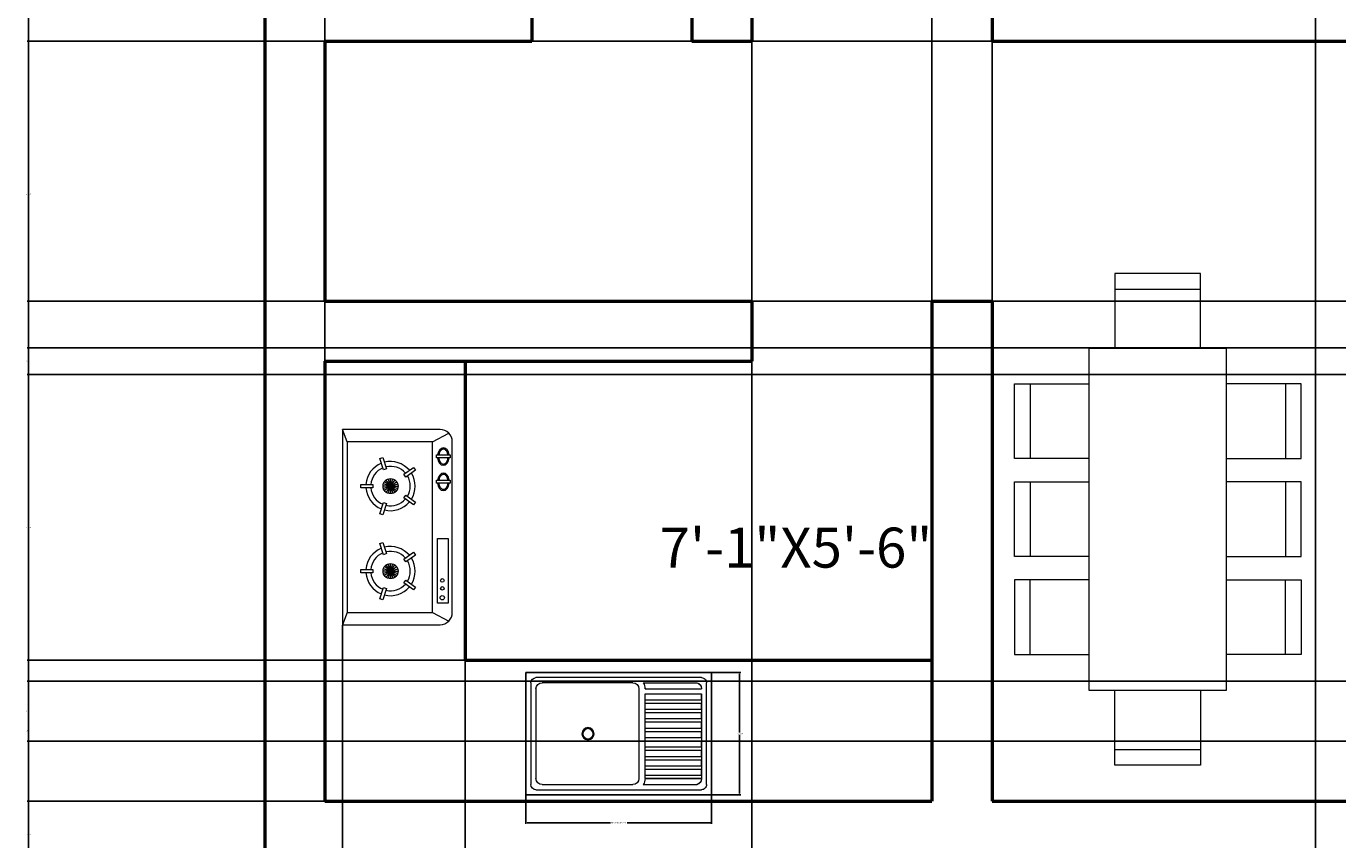
# Model space of a CAD drawing. Units: inches. Extents: x 3 to 576, y -689 to 51.
# Tile 6 of 21: x 3 to 199, y -383 to -261. Entities that reach past the tile are written whole.
import ezdxf

# ---------------------------------------------------------------- set-up
doc = ezdxf.new("R2010")
doc.units = ezdxf.units.IN
doc.header["$MEASUREMENT"] = 0
for name, color, linetype, lineweight in [('A-ANNO-DIMS', 2, 'Continuous', 18), ('A-AREA-IDEN', 7, 'Continuous', 18), ('A-EQPM', 8, 'Continuous', 18), ('A-FLOR-FIXT', 9, 'Continuous', 18), ('A-FURN', 8, 'Continuous', 18), ('A-WALL', 7, 'Continuous', 50)]:
    doc.layers.add(name, color=color, linetype=linetype, lineweight=lineweight)
doc.styles.get("Standard").update_dxf_attribs({"font": 'arial.ttf'})
doc.dimstyles.get("Standard").update_dxf_attribs({"dimtxt": 0.18, "dimasz": 0.18, "dimexe": 0.18, "dimexo": 0.0625, "dimgap": 0.09, "dimtad": 0, "dimtih": 1, "dimtoh": 1, "dimdec": 0, "dimzin": 0, "dimdsep": 46, "dimlunit": 3, "dimtxsty": 'Standard', "dimcen": 0.09, "dimadec": 0, "dimazin": 0, "dimtfac": 1, "dimtdec": 0, "dimtofl": 0, "dimtmove": 0, "dimatfit": 3, "dimfxl": 1, "dimtolj": 1, "dimtzin": 0, "dimarcsym": 0})

# ---------------------------------------------------------------- blocks, each defined once
blk = doc.blocks.new('М12 540х820')
for p, q in [((0, 540), (-820, 540)), ((-820, 540), (-820, 0)), ((0, 0), (0, 540)), ((-797.5, 495), (-797.5, 45)), ((-45, 517.5), (-775, 517.5)), ((-775, 468), (-775, 72)), ((-347.5, 495), (-748, 495)), ((-320.5, 468), (-320.5, 72)), ((-301.7, 495), (-64.8, 495)), ((-293.7, 468), (-293.7, 472.5)), ((-293.7, 468), (-45, 468)), ((-45, 469.5), (-45, 468)), ((-22.5, 45), (-22.5, 495)), ((-293.7, 446.6), (-45, 446.6)), ((-293.7, 419.6), (-293.7, 446.6)), ((-293.7, 419.6), (-45, 419.6)), ((-45, 419.6), (-45, 446.6)), ((-293.7, 405), (-45, 405)), ((-293.7, 378), (-293.7, 405)), ((-293.7, 378), (-45, 378)), ((-293.7, 336.4), (-293.7, 363.4)), ((-293.7, 363.4), (-45, 363.4)), ((-45, 378), (-45, 405)), ((-45, 336.4), (-45, 363.4)), ((-293.7, 336.4), (-45, 336.4)), ((-293.7, 294.7), (-293.7, 321.7)), ((-293.7, 321.7), (-45, 321.7)), ((-293.7, 294.7), (-45, 294.7)), ((-45, 294.7), (-45, 321.7)), ((-293.7, 253.1), (-293.7, 280.1)), ((-293.7, 280.1), (-45, 280.1)), ((-293.7, 253.1), (-45, 253.1)), ((-293.7, 211.5), (-293.7, 238.5)), ((-293.7, 238.5), (-45, 238.5)), ((-45, 253.1), (-45, 280.1)), ((-45, 211.5), (-45, 238.5)), ((-293.7, 211.5), (-45, 211.5)), ((-293.7, 169.9), (-293.7, 196.9)), ((-293.7, 196.9), (-45, 196.9)), ((-45, 169.9), (-45, 196.9)), ((-293.7, 169.9), (-45, 169.9)), ((-293.7, 128.2), (-293.7, 155.2)), ((-293.7, 155.2), (-45, 155.2)), ((-293.7, 128.2), (-45, 128.2)), ((-45, 128.2), (-45, 155.2)), ((-293.7, 113.6), (-45, 113.6)), ((-293.7, 86.6), (-293.7, 113.6)), ((-293.7, 86.6), (-45, 86.6)), ((-293.7, 72), (-45, 72)), ((-45, 86.6), (-45, 113.6)), ((-45, 70.5), (-45, 72)), ((-820, 0), (0, 0)), ((-775, 22.5), (-45, 22.5)), ((-748, 45), (-347.5, 45)), ((-301.7, 45), (-64.8, 45))]:
    blk.add_line(p, q)
at = {"ltscale": 0.06}
for p, q in [((-820, 0), (-820, 540)), ((-820, 540), (0, 540)), ((0, 540), (0, 536.9)), ((0, 536.9), (0, 0)), ((-293.7, 446.6), (-45, 446.6)), ((-293.7, 405), (-293.7, 446.6)), ((-45, 446.6), (-45, 419.6)), ((-45, 419.6), (-45, 378)), ((-293.7, 363.4), (-293.7, 405)), ((-293.7, 321.7), (-293.7, 363.4)), ((-45, 378), (-45, 336.4)), ((-293.7, 280.1), (-293.7, 321.7)), ((-45, 336.4), (-45, 294.7)), ((-45, 294.7), (-45, 253.1)), ((-293.7, 238.5), (-293.7, 280.1)), ((-293.7, 196.9), (-293.7, 238.5)), ((-45, 253.1), (-45, 211.5)), ((-293.7, 155.2), (-293.7, 196.9)), ((-45, 211.5), (-45, 169.9)), ((-293.7, 113.6), (-293.7, 155.2)), ((-45, 169.9), (-45, 128.2)), ((-45, 128.2), (-45, 86.6)), ((-293.7, 72), (-293.7, 113.6)), ((-45, 72), (-293.7, 72)), ((-45, 86.6), (-45, 72)), ((0, 0), (-820, 0))]:
    blk.add_line(p, q, dxfattribs=at)
at = {"extrusion": (0, 0, -1)}
for centre, major_axis, start_param, end_param in [((-775, 495), (-15.9, 15.9), -0.785398, 0.785398), ((-775, 495), (-15.9, 15.9), -0.785398, 0.785398), ((-748, 468), (-19.1, -19.1), 0.785398, 2.356194), ((-748, 468), (-19.1, -19.1), 0.785398, 2.356194), ((-347.5, 468), (-19.1, 19.1), 0.785398, 2.356194), ((-347.5, 468), (-19.1, 19.1), 0.785398, 2.356194), ((-343.2, 468), (-35, 35), 1.779263, 2.356194), ((-343.2, 468), (-35, 35), 1.779263, 2.356192), ((-343.2, 468), (-35, 35), 2.356192, 2.356194), ((-72.3, 468.8), (-19.3, 19.3), 1.0328, 2.38382), ((-72.3, 468.8), (-19.3, 19.3), 1.0328, 1.064673), ((-72.3, 468.8), (-19.3, 19.3), 1.064673, 2.328569), ((-45, 495), (-15.9, -15.9), 2.356194, 3.926991), ((-45, 495), (-15.9, -15.9), 2.356194, 3.926991), ((-72.3, 468.8), (-19.3, 19.3), 2.328569, 2.38382), ((-545.5, 270), (-19.1, -19.1), 3.926991, 10.210176), ((-545.5, 270), (-19.1, -19.1), 3.926991, 10.210176), ((-545.5, 270), (-15.9, -15.9), 3.926991, 10.210176), ((-545.5, 270), (-15.9, -15.9), 3.926991, 10.210176), ((-748, 72), (-19.1, 19.1), 3.926991, 5.497787), ((-748, 72), (-19.1, 19.1), 3.926991, 5.497787), ((-347.5, 72), (-19.1, -19.1), 3.926991, 5.497787), ((-347.5, 72), (-19.1, -19.1), 3.926991, 5.497787), ((-343.2, 72), (-35, -35), 3.926991, 4.503922), ((-343.2, 72), (-35, -35), 3.926991, 4.503922), ((-72.3, 71.2), (-19.3, -19.3), 3.899365, 5.250385), ((-72.3, 71.2), (-19.3, -19.3), 3.954617, 5.218512), ((-72.3, 71.2), (-19.3, -19.3), 3.899365, 3.954617), ((-775, 45), (-15.9, -15.9), 5.497787, 7.068583), ((-775, 45), (-15.9, -15.9), 5.497787, 7.068583), ((-72.3, 71.2), (-19.3, -19.3), 5.218512, 5.250385), ((-45, 45), (-15.9, 15.9), 2.356194, 3.926991), ((-45, 45), (-15.9, 15.9), 2.356194, 3.926991)]:
    blk.add_ellipse(centre, major_axis=major_axis, ratio=1, start_param=start_param, end_param=end_param, dxfattribs=at)
blk = doc.blocks.new('*D23')
at = {"layer": 'A-ANNO-DIMS', "color": 0, "lineweight": -2, "transparency": 16777216}
for p, q in [((77.4, -376.43), (77.4, -380.72)), ((105.25, -376.43), (105.25, -380.72)), ((77.58, -380.54), (90.08, -380.54)), ((105.07, -380.54), (92.57, -380.54))]:
    blk.add_line(p, q, dxfattribs=at)
at = {"layer": 'A-ANNO-DIMS', "color": 0, "transparency": 16777216}
for points in [[(77.58, -380.51), (77.58, -380.57), (77.4, -380.54)], [(105.07, -380.51), (105.07, -380.57), (105.25, -380.54)]]:
    blk.add_solid(points, dxfattribs=at)
at = {"layer": 'Defpoints', "color": 0, "transparency": 16777216}
for p in [(77.4, -376.36), (105.25, -376.36), (105.25, -380.54)]:
    blk.add_point(p, dxfattribs=at)
at = {"layer": 'A-ANNO-DIMS', "color": 0, "transparency": 16777216, "insert": (91.33, -380.54), "char_height": 0.18, "attachment_point": 5}
blk.add_mtext('\\A1;KITCHEN SINK 2\'-4"', dxfattribs=at)
blk = doc.blocks.new('*D24')
at = {"layer": 'A-ANNO-DIMS', "color": 0, "lineweight": -2, "transparency": 16777216}
for p, q in [((105.31, -358.02), (109.61, -358.02)), ((109.43, -358.2), (109.43, -367.01)), ((109.43, -376.18), (109.43, -367.38)), ((105.31, -376.36), (109.61, -376.36))]:
    blk.add_line(p, q, dxfattribs=at)
at = {"layer": 'A-ANNO-DIMS', "color": 0, "transparency": 16777216}
for points in [[(109.4, -358.2), (109.46, -358.2), (109.43, -358.02)], [(109.4, -376.18), (109.46, -376.18), (109.43, -376.36)]]:
    blk.add_solid(points, dxfattribs=at)
at = {"layer": 'Defpoints', "color": 0, "transparency": 16777216}
for p in [(105.25, -358.02), (109.43, -358.02), (105.25, -376.36)]:
    blk.add_point(p, dxfattribs=at)
at = {"layer": 'A-ANNO-DIMS', "color": 0, "transparency": 16777216, "insert": (109.43, -367.19), "char_height": 0.18, "attachment_point": 5}
blk.add_mtext('\\A1;1\'-6 1/2"', dxfattribs=at)
blk = doc.blocks.new('*D57')
at = {"layer": 'A-ANNO-DIMS', "color": 0, "lineweight": -2, "transparency": 16777216}
for p, q in [((38.23, -178.31), (2.66, -178.31)), ((2.84, -178.49), (2.84, -240.13)), ((2.84, -302.13), (2.84, -240.49)), ((47.23, -302.31), (2.66, -302.31))]:
    blk.add_line(p, q, dxfattribs=at)
at = {"layer": 'A-ANNO-DIMS', "color": 0, "transparency": 16777216}
for points in [[(2.81, -178.49), (2.87, -178.49), (2.84, -178.31)], [(2.81, -302.13), (2.87, -302.13), (2.84, -302.31)]]:
    blk.add_solid(points, dxfattribs=at)
at = {"layer": 'Defpoints', "color": 0, "transparency": 16777216}
for p in [(38.29, -178.31), (2.84, -302.31), (47.29, -302.31)]:
    blk.add_point(p, dxfattribs=at)
at = {"layer": 'A-ANNO-DIMS', "color": 0, "transparency": 16777216, "insert": (2.84, -240.31), "char_height": 0.18, "attachment_point": 5}
blk.add_mtext('\\A1;10\'-4"', dxfattribs=at)
blk = doc.blocks.new('*D58')
at = {"layer": 'A-ANNO-DIMS', "color": 0, "lineweight": -2, "transparency": 16777216}
for p, q in [((47.23, -302.31), (2.66, -302.31)), ((2.84, -302.49), (2.84, -382.13)), ((2.84, -462.13), (2.84, -382.49)), ((38.23, -462.31), (2.66, -462.31))]:
    blk.add_line(p, q, dxfattribs=at)
at = {"layer": 'A-ANNO-DIMS', "color": 0, "transparency": 16777216}
for points in [[(2.81, -302.49), (2.87, -302.49), (2.84, -302.31)], [(2.81, -462.13), (2.87, -462.13), (2.84, -462.31)]]:
    blk.add_solid(points, dxfattribs=at)
at = {"layer": 'Defpoints', "color": 0, "transparency": 16777216}
for p in [(47.29, -302.31), (2.84, -462.31), (38.29, -462.31)]:
    blk.add_point(p, dxfattribs=at)
at = {"layer": 'A-ANNO-DIMS', "color": 0, "transparency": 16777216, "insert": (2.84, -382.31), "char_height": 0.18, "attachment_point": 5}
blk.add_mtext('\\A1;13\'-4"', dxfattribs=at)
blk = doc.blocks.new('*D63')
at = {"layer": 'A-ANNO-DIMS', "color": 0, "lineweight": -2, "transparency": 16777216}
for p, q in [((47.36, -263.31), (575.92, -263.31)), ((575.74, -263.49), (575.74, -282.63)), ((575.74, -302.13), (575.74, -282.99)), ((47.36, -302.31), (575.92, -302.31))]:
    blk.add_line(p, q, dxfattribs=at)
at = {"layer": 'A-ANNO-DIMS', "color": 0, "transparency": 16777216}
for points in [[(575.71, -263.49), (575.77, -263.49), (575.74, -263.31)], [(575.71, -302.13), (575.77, -302.13), (575.74, -302.31)]]:
    blk.add_solid(points, dxfattribs=at)
at = {"layer": 'Defpoints', "color": 0, "transparency": 16777216}
for p in [(47.29, -263.31), (47.29, -302.31), (575.74, -302.31)]:
    blk.add_point(p, dxfattribs=at)
at = {"layer": 'A-ANNO-DIMS', "color": 0, "transparency": 16777216, "insert": (575.74, -282.81), "char_height": 0.18, "attachment_point": 5}
blk.add_mtext('\\A1;3\'-3"', dxfattribs=at)
blk = doc.blocks.new('*D68')
at = {"layer": 'A-ANNO-DIMS', "color": 0, "lineweight": -2, "transparency": 16777216}
for p, q in [((531.23, -254.31), (2.66, -254.31)), ((2.84, -254.49), (2.84, -258.63)), ((2.84, -263.13), (2.84, -258.99)), ((531.23, -263.31), (2.66, -263.31))]:
    blk.add_line(p, q, dxfattribs=at)
at = {"layer": 'A-ANNO-DIMS', "color": 0, "transparency": 16777216}
for points in [[(2.81, -254.49), (2.87, -254.49), (2.84, -254.31)], [(2.81, -263.13), (2.87, -263.13), (2.84, -263.31)]]:
    blk.add_solid(points, dxfattribs=at)
at = {"layer": 'Defpoints', "color": 0, "transparency": 16777216}
for p in [(531.29, -254.31), (2.84, -263.31), (531.29, -263.31)]:
    blk.add_point(p, dxfattribs=at)
at = {"layer": 'A-ANNO-DIMS', "color": 0, "transparency": 16777216, "insert": (2.84, -258.81), "char_height": 0.18, "attachment_point": 5}
blk.add_mtext('\\A1;0\'-9"', dxfattribs=at)
blk = doc.blocks.new('*D69')
at = {"layer": 'A-ANNO-DIMS', "color": 0, "lineweight": -2, "transparency": 16777216}
for p, q in [((531.23, -263.31), (2.66, -263.31)), ((2.84, -263.49), (2.84, -311.13)), ((2.84, -359.13), (2.84, -311.49)), ((531.23, -359.31), (2.66, -359.31))]:
    blk.add_line(p, q, dxfattribs=at)
at = {"layer": 'A-ANNO-DIMS', "color": 0, "transparency": 16777216}
for points in [[(2.81, -263.49), (2.87, -263.49), (2.84, -263.31)], [(2.81, -359.13), (2.87, -359.13), (2.84, -359.31)]]:
    blk.add_solid(points, dxfattribs=at)
at = {"layer": 'Defpoints', "color": 0, "transparency": 16777216}
for p in [(531.29, -263.31), (2.84, -359.31), (531.29, -359.31)]:
    blk.add_point(p, dxfattribs=at)
at = {"layer": 'A-ANNO-DIMS', "color": 0, "transparency": 16777216, "insert": (2.84, -311.31), "char_height": 0.18, "attachment_point": 5}
blk.add_mtext('\\A1;8\'-0"', dxfattribs=at)
blk = doc.blocks.new('*D70')
at = {"layer": 'A-ANNO-DIMS', "color": 0, "lineweight": -2, "transparency": 16777216}
for p, q in [((531.23, -359.31), (2.66, -359.31)), ((2.84, -359.49), (2.84, -363.63)), ((2.84, -368.13), (2.84, -363.99)), ((531.23, -368.31), (2.66, -368.31))]:
    blk.add_line(p, q, dxfattribs=at)
at = {"layer": 'A-ANNO-DIMS', "color": 0, "transparency": 16777216}
for points in [[(2.81, -359.49), (2.87, -359.49), (2.84, -359.31)], [(2.81, -368.13), (2.87, -368.13), (2.84, -368.31)]]:
    blk.add_solid(points, dxfattribs=at)
at = {"layer": 'Defpoints', "color": 0, "transparency": 16777216}
for p in [(531.29, -359.31), (2.84, -368.31), (531.29, -368.31)]:
    blk.add_point(p, dxfattribs=at)
at = {"layer": 'A-ANNO-DIMS', "color": 0, "transparency": 16777216, "insert": (2.84, -363.81), "char_height": 0.18, "attachment_point": 5}
blk.add_mtext('\\A1;0\'-9"', dxfattribs=at)
blk = doc.blocks.new('*D71')
at = {"layer": 'A-ANNO-DIMS', "color": 0, "lineweight": -2, "transparency": 16777216}
for p, q in [((531.23, -368.31), (2.66, -368.31)), ((2.84, -368.49), (2.84, -404.13)), ((2.84, -440.13), (2.84, -404.49)), ((531.23, -440.31), (2.66, -440.31))]:
    blk.add_line(p, q, dxfattribs=at)
at = {"layer": 'A-ANNO-DIMS', "color": 0, "transparency": 16777216}
for points in [[(2.81, -368.49), (2.87, -368.49), (2.84, -368.31)], [(2.81, -440.13), (2.87, -440.13), (2.84, -440.31)]]:
    blk.add_solid(points, dxfattribs=at)
at = {"layer": 'Defpoints', "color": 0, "transparency": 16777216}
for p in [(531.29, -368.31), (2.84, -440.31), (531.29, -440.31)]:
    blk.add_point(p, dxfattribs=at)
at = {"layer": 'A-ANNO-DIMS', "color": 0, "transparency": 16777216, "insert": (2.84, -404.31), "char_height": 0.18, "attachment_point": 5}
blk.add_mtext('\\A1;6\'-0"', dxfattribs=at)
blk = doc.blocks.new('*D84')
at = {"layer": 'A-ANNO-DIMS', "color": 0, "lineweight": -2, "transparency": 16777216}
for p, q in [((385.3, -263.31), (2.66, -263.31)), ((2.84, -263.49), (2.84, -286.13)), ((2.84, -309.13), (2.84, -286.49)), ((385.3, -309.31), (2.66, -309.31))]:
    blk.add_line(p, q, dxfattribs=at)
at = {"layer": 'A-ANNO-DIMS', "color": 0, "transparency": 16777216}
for points in [[(2.81, -263.49), (2.87, -263.49), (2.84, -263.31)], [(2.81, -309.13), (2.87, -309.13), (2.84, -309.31)]]:
    blk.add_solid(points, dxfattribs=at)
at = {"layer": 'Defpoints', "color": 0, "transparency": 16777216}
for p in [(385.37, -263.31), (2.84, -309.31), (385.37, -309.31)]:
    blk.add_point(p, dxfattribs=at)
at = {"layer": 'A-ANNO-DIMS', "color": 0, "transparency": 16777216, "insert": (2.84, -286.31), "char_height": 0.18, "attachment_point": 5}
blk.add_mtext('\\A1;3\'-10"', dxfattribs=at)
blk = doc.blocks.new('*D85')
at = {"layer": 'A-ANNO-DIMS', "color": 0, "lineweight": -2, "transparency": 16777216}
for p, q in [((385.3, -313.31), (2.66, -313.31)), ((2.84, -313.49), (2.84, -336.13)), ((2.84, -359.13), (2.84, -336.49)), ((385.3, -359.31), (2.66, -359.31))]:
    blk.add_line(p, q, dxfattribs=at)
at = {"layer": 'A-ANNO-DIMS', "color": 0, "transparency": 16777216}
for points in [[(2.81, -313.49), (2.87, -313.49), (2.84, -313.31)], [(2.81, -359.13), (2.87, -359.13), (2.84, -359.31)]]:
    blk.add_solid(points, dxfattribs=at)
at = {"layer": 'Defpoints', "color": 0, "transparency": 16777216}
for p in [(385.37, -313.31), (2.84, -359.31), (385.37, -359.31)]:
    blk.add_point(p, dxfattribs=at)
at = {"layer": 'A-ANNO-DIMS', "color": 0, "transparency": 16777216, "insert": (2.84, -336.31), "char_height": 0.18, "attachment_point": 5}
blk.add_mtext('\\A1;3\'-10"', dxfattribs=at)
blk = doc.blocks.new('*D86')
at = {"layer": 'A-ANNO-DIMS', "color": 0, "lineweight": -2, "transparency": 16777216}
for p, q in [((111.29, -97.21), (111.29, -688.94)), ((195.78, -97.21), (195.78, -688.94)), ((111.47, -688.76), (153, -688.76)), ((195.6, -688.76), (154.08, -688.76))]:
    blk.add_line(p, q, dxfattribs=at)
at = {"layer": 'A-ANNO-DIMS', "color": 0, "transparency": 16777216}
for points in [[(111.47, -688.73), (111.47, -688.79), (111.29, -688.76)], [(195.6, -688.73), (195.6, -688.79), (195.78, -688.76)]]:
    blk.add_solid(points, dxfattribs=at)
at = {"layer": 'Defpoints', "color": 0, "transparency": 16777216}
for p in [(111.29, -97.15), (195.78, -97.15), (195.78, -688.76)]:
    blk.add_point(p, dxfattribs=at)
at = {"layer": 'A-ANNO-DIMS', "color": 0, "transparency": 16777216, "insert": (153.54, -688.76), "char_height": 0.18, "attachment_point": 5}
blk.add_mtext('\\A1;7\'-0 1/2"', dxfattribs=at)
blk = doc.blocks.new('*D114')
at = {"layer": 'A-ANNO-DIMS', "color": 0, "lineweight": -2, "transparency": 16777216}
for p, q in [((147.29, -377.25), (147.29, 51.32)), ((147.47, 51.14), (182.96, 51.14)), ((219.11, 51.14), (183.62, 51.14)), ((219.29, -377.25), (219.29, 51.32))]:
    blk.add_line(p, q, dxfattribs=at)
at = {"layer": 'A-ANNO-DIMS', "color": 0, "transparency": 16777216}
for points in [[(147.47, 51.17), (147.47, 51.11), (147.29, 51.14)], [(219.11, 51.17), (219.11, 51.11), (219.29, 51.14)]]:
    blk.add_solid(points, dxfattribs=at)
at = {"layer": 'Defpoints', "color": 0, "transparency": 16777216}
for p in [(219.29, 51.14), (147.29, -377.31), (219.29, -377.31)]:
    blk.add_point(p, dxfattribs=at)
at = {"layer": 'A-ANNO-DIMS', "color": 0, "transparency": 16777216, "insert": (183.29, 51.14), "char_height": 0.18, "attachment_point": 5}
blk.add_mtext('\\A1;6\'-0"', dxfattribs=at)
blk = doc.blocks.new('*D119')
at = {"layer": 'A-ANNO-DIMS', "color": 0, "lineweight": -2, "transparency": 16777216}
for p, q in [((47.29, -311.25), (47.29, 51.32)), ((47.47, 51.14), (78.96, 51.14)), ((111.11, 51.14), (79.62, 51.14)), ((111.29, -311.25), (111.29, 51.32))]:
    blk.add_line(p, q, dxfattribs=at)
at = {"layer": 'A-ANNO-DIMS', "color": 0, "transparency": 16777216}
for points in [[(47.47, 51.17), (47.47, 51.11), (47.29, 51.14)], [(111.11, 51.17), (111.11, 51.11), (111.29, 51.14)]]:
    blk.add_solid(points, dxfattribs=at)
at = {"layer": 'Defpoints', "color": 0, "transparency": 16777216}
for p in [(111.29, 51.14), (47.29, -311.31), (111.29, -311.31)]:
    blk.add_point(p, dxfattribs=at)
at = {"layer": 'A-ANNO-DIMS', "color": 0, "transparency": 16777216, "insert": (79.29, 51.14), "char_height": 0.18, "attachment_point": 5}
blk.add_mtext('\\A1;5\'-4"', dxfattribs=at)
blk = doc.blocks.new('*D120')
at = {"layer": 'A-ANNO-DIMS', "color": 0, "lineweight": -2, "transparency": 16777216}
for p, q in [((111.29, -302.25), (111.29, 51.32)), ((111.47, 51.14), (124.46, 51.14)), ((138.11, 51.14), (125.12, 51.14)), ((138.29, -302.25), (138.29, 51.32))]:
    blk.add_line(p, q, dxfattribs=at)
at = {"layer": 'A-ANNO-DIMS', "color": 0, "transparency": 16777216}
for points in [[(111.47, 51.17), (111.47, 51.11), (111.29, 51.14)], [(138.11, 51.17), (138.11, 51.11), (138.29, 51.14)]]:
    blk.add_solid(points, dxfattribs=at)
at = {"layer": 'Defpoints', "color": 0, "transparency": 16777216}
for p in [(138.29, 51.14), (111.29, -302.31), (138.29, -302.31)]:
    blk.add_point(p, dxfattribs=at)
at = {"layer": 'A-ANNO-DIMS', "color": 0, "transparency": 16777216, "insert": (124.79, 51.14), "char_height": 0.18, "attachment_point": 5}
blk.add_mtext('\\A1;2\'-3"', dxfattribs=at)
blk = doc.blocks.new('*D121')
at = {"layer": 'A-ANNO-DIMS', "color": 0, "lineweight": -2, "transparency": 16777216}
for p, q in [((49.91, -350.9), (49.91, -688.94)), ((68.33, -356.2), (68.33, -688.94)), ((50.09, -688.76), (58.59, -688.76)), ((68.15, -688.76), (59.65, -688.76))]:
    blk.add_line(p, q, dxfattribs=at)
at = {"layer": 'A-ANNO-DIMS', "color": 0, "transparency": 16777216}
for points in [[(50.09, -688.73), (50.09, -688.79), (49.91, -688.76)], [(68.15, -688.73), (68.15, -688.79), (68.33, -688.76)]]:
    blk.add_solid(points, dxfattribs=at)
at = {"layer": 'Defpoints', "color": 0, "transparency": 16777216}
for p in [(49.91, -350.84), (68.33, -356.14), (68.33, -688.76)]:
    blk.add_point(p, dxfattribs=at)
at = {"layer": 'A-ANNO-DIMS', "color": 0, "transparency": 16777216, "insert": (59.12, -688.76), "char_height": 0.18, "attachment_point": 5}
blk.add_mtext('\\A1;1\'-6 1/2"', dxfattribs=at)
blk = doc.blocks.new('*D122')
at = {"layer": 'A-ANNO-DIMS', "color": 0, "lineweight": -2, "transparency": 16777216}
for p, q in [((138.23, -356.14), (2.66, -356.14)), ((2.84, -356.32), (2.84, -366.54)), ((2.84, -377.13), (2.84, -366.91)), ((138.23, -377.31), (2.66, -377.31))]:
    blk.add_line(p, q, dxfattribs=at)
at = {"layer": 'A-ANNO-DIMS', "color": 0, "transparency": 16777216}
for points in [[(2.81, -356.32), (2.87, -356.32), (2.84, -356.14)], [(2.81, -377.13), (2.87, -377.13), (2.84, -377.31)]]:
    blk.add_solid(points, dxfattribs=at)
at = {"layer": 'Defpoints', "color": 0, "transparency": 16777216}
for p in [(138.29, -356.14), (2.84, -377.31), (138.29, -377.31)]:
    blk.add_point(p, dxfattribs=at)
at = {"layer": 'A-ANNO-DIMS', "color": 0, "transparency": 16777216, "insert": (2.84, -366.72), "char_height": 0.18, "attachment_point": 5}
blk.add_mtext('\\A1;1\'-9"', dxfattribs=at)
blk = doc.blocks.new('*D125')
at = {"layer": 'A-ANNO-DIMS', "color": 0, "lineweight": -2, "transparency": 16777216}
for p, q in [((531.23, -368.31), (2.66, -368.31)), ((2.84, -368.49), (2.84, -377.13)), ((2.84, -386.13), (2.84, -377.49)), ((512.45, -386.31), (2.66, -386.31))]:
    blk.add_line(p, q, dxfattribs=at)
at = {"layer": 'A-ANNO-DIMS', "color": 0, "transparency": 16777216}
for points in [[(2.81, -368.49), (2.87, -368.49), (2.84, -368.31)], [(2.81, -386.13), (2.87, -386.13), (2.84, -386.31)]]:
    blk.add_solid(points, dxfattribs=at)
at = {"layer": 'Defpoints', "color": 0, "transparency": 16777216}
for p in [(531.29, -368.31), (2.84, -386.31), (512.51, -386.31)]:
    blk.add_point(p, dxfattribs=at)
at = {"layer": 'A-ANNO-DIMS', "color": 0, "transparency": 16777216, "insert": (2.84, -377.31), "char_height": 0.18, "attachment_point": 5}
blk.add_mtext('\\A1;1\'-6"', dxfattribs=at)

msp = doc.modelspace()

# ---------------------------------------------------------------- linework, layer by layer
at = {"layer": 'A-EQPM'}
for p, q in [((64.55, -321.57), (49.91, -321.57)), ((49.91, -321.57), (49.91, -350.84)), ((50.61, -323.4), (49.91, -321.57)), ((63.41, -323.4), (65.84, -322.1)), ((63.41, -323.4), (50.61, -323.4)), ((50.61, -323.4), (50.61, -349.01)), ((63.41, -349.01), (63.41, -323.4)), ((66.38, -349.01), (66.38, -323.4)), ((55.51, -325.9), (55.98, -325.75)), ((56.06, -327.59), (55.51, -325.9)), ((55.98, -325.75), (56.53, -327.44)), ((64.02, -325.83), (64.02, -325.36)), ((64.02, -325.36), (66.05, -325.36)), ((66.05, -325.83), (64.02, -325.83)), ((66.05, -325.36), (66.05, -325.83)), ((56.53, -327.44), (56.06, -327.59)), ((59.13, -328.28), (60.57, -327.24)), ((59.42, -328.69), (59.13, -328.28)), ((60.86, -327.64), (59.42, -328.69)), ((60.57, -327.24), (60.86, -327.64)), ((52.67, -330.3), (52.67, -329.8)), ((52.67, -329.8), (54.45, -329.8)), ((54.45, -330.3), (52.67, -330.3)), ((54.45, -329.8), (54.45, -330.3)), ((57.12, -330.05), (55.99, -330.05)), ((57.12, -330.05), (56.05, -329.71)), ((57.12, -330.05), (56.05, -330.4)), ((57.12, -330.05), (56.21, -329.39)), ((57.12, -330.05), (56.21, -330.72)), ((57.12, -330.05), (56.46, -329.14)), ((57.12, -330.05), (56.46, -330.97)), ((57.12, -330.05), (56.77, -328.98)), ((57.12, -330.05), (56.77, -331.13)), ((57.12, -330.05), (57.12, -328.93)), ((57.12, -330.05), (57.47, -328.98)), ((57.12, -330.05), (57.78, -329.14)), ((57.12, -330.05), (58.03, -329.39)), ((57.12, -330.05), (58.19, -329.71)), ((57.12, -330.05), (58.24, -330.05)), ((57.12, -330.05), (58.19, -330.4)), ((57.12, -330.05), (58.03, -330.72)), ((57.12, -330.05), (57.78, -330.97)), ((57.12, -330.05), (57.47, -331.13)), ((57.12, -330.05), (57.12, -331.18)), ((64.02, -329.15), (66.05, -329.15)), ((64.02, -329.62), (64.02, -329.15)), ((66.05, -329.62), (64.02, -329.62)), ((66.05, -329.15), (66.05, -329.62)), ((59.13, -331.82), (59.42, -331.42)), ((60.57, -332.87), (59.13, -331.82)), ((59.42, -331.42), (60.86, -332.46)), ((55.51, -334.2), (56.06, -332.51)), ((55.98, -334.36), (55.51, -334.2)), ((56.53, -332.67), (55.98, -334.36)), ((56.06, -332.51), (56.53, -332.67)), ((60.86, -332.46), (60.57, -332.87)), ((64.18, -347.61), (64.18, -337.93)), ((64.18, -337.93), (65.75, -337.93)), ((65.75, -337.93), (65.75, -347.61)), ((55.51, -338.65), (55.98, -338.49)), ((56.06, -340.34), (55.51, -338.65)), ((55.98, -338.49), (56.53, -340.18)), ((59.13, -341.03), (60.57, -339.98)), ((60.57, -339.98), (60.86, -340.39)), ((56.53, -340.18), (56.06, -340.34)), ((57.12, -342.8), (56.46, -341.88)), ((57.12, -342.8), (56.77, -341.72)), ((57.12, -342.8), (57.12, -341.67)), ((57.12, -342.8), (57.47, -341.72)), ((57.12, -342.8), (57.78, -341.88)), ((59.42, -341.43), (59.13, -341.03)), ((60.86, -340.39), (59.42, -341.43)), ((52.67, -343.05), (52.67, -342.55)), ((52.67, -342.55), (54.45, -342.55)), ((54.45, -343.05), (52.67, -343.05)), ((54.45, -342.55), (54.45, -343.05)), ((57.12, -342.8), (55.99, -342.8)), ((57.12, -342.8), (56.05, -342.45)), ((57.12, -342.8), (56.05, -343.14)), ((57.12, -342.8), (56.21, -342.13)), ((57.12, -342.8), (56.21, -343.46)), ((57.12, -342.8), (56.46, -343.71)), ((57.12, -342.8), (56.77, -343.87)), ((57.12, -342.8), (58.03, -342.13)), ((57.12, -342.8), (58.19, -342.45)), ((57.12, -342.8), (57.12, -343.92)), ((57.12, -342.8), (57.47, -343.87)), ((57.12, -342.8), (57.78, -343.71)), ((57.12, -342.8), (58.03, -343.46)), ((57.12, -342.8), (58.19, -343.14)), ((57.12, -342.8), (58.24, -342.8)), ((55.51, -346.94), (56.06, -345.25)), ((56.53, -345.41), (55.98, -347.1)), ((56.06, -345.25), (56.53, -345.41)), ((59.13, -344.57), (59.42, -344.16)), ((60.57, -345.61), (59.13, -344.57)), ((59.42, -344.16), (60.86, -345.21)), ((60.86, -345.21), (60.57, -345.61)), ((55.98, -347.1), (55.51, -346.94)), ((65.75, -347.61), (64.18, -347.61)), ((50.61, -349.01), (49.91, -350.84)), ((50.61, -349.01), (63.41, -349.01)), ((63.41, -349.01), (65.84, -350.31)), ((49.91, -350.84), (64.55, -350.84))]:
    msp.add_line(p, q, dxfattribs=at)
for centre, radius in [((57.12, -330.05), 1.13), ((57.12, -342.8), 1.13), ((64.88, -344.2), 0.27), ((64.88, -345.39), 0.27), ((64.88, -346.8), 0.324)]:
    msp.add_circle(centre, radius, dxfattribs=at)
for centre, radius, start, end in [((64.55, -323.4), 1.83, 0, 90), ((57.12, -330.05), 3.69, 39.8765, 104.1235), ((57.12, -330.05), 3.69, 111.8765, 176.1235), ((57.12, -330.05), 2.96, 112.8365, 175.1635), ((57.12, -330.05), 2.96, 40.8365, 103.1635), ((57.12, -330.05), 3.69, 327.8765, 32.1235), ((57.12, -330.05), 3.69, 183.8765, 248.1235), ((57.12, -330.05), 2.96, 184.8365, 247.1635), ((57.12, -330.05), 2.96, 328.8365, 31.1635), ((57.12, -330.05), 2.96, 256.8365, 319.1635), ((57.12, -330.05), 3.69, 255.8765, 320.1235), ((57.12, -342.8), 3.69, 111.8765, 176.1235), ((57.12, -342.8), 2.96, 112.8365, 175.1635), ((57.12, -342.8), 3.69, 39.8765, 104.1235), ((57.12, -342.8), 2.96, 40.8365, 103.1635), ((57.12, -342.8), 2.96, 328.8365, 31.1635), ((57.12, -342.8), 3.69, 327.8765, 32.1235), ((57.12, -342.8), 3.69, 183.8765, 248.1235), ((57.12, -342.8), 2.96, 184.8365, 247.1635), ((57.12, -342.8), 3.69, 255.8765, 320.1235), ((57.12, -342.8), 2.96, 256.8365, 319.1635), ((64.55, -349.01), 1.83, 270, 0)]:
    msp.add_arc(centre, radius, start, end, dxfattribs=at)
for centre, major_axis, start_param, end_param in [((65.04, -325.62), (0, -1.31), 1.774361, 4.508825), ((65.04, -325.62), (0, 1.31), 1.73081, 4.552375), ((65.04, -329.41), (0, -1.31), 1.774361, 4.508825), ((65.04, -329.41), (0, 1.31), 1.73081, 4.552375)]:
    msp.add_ellipse(centre, major_axis=major_axis, ratio=0.671641, start_param=start_param, end_param=end_param, dxfattribs=at)
for points, knots in [([(64.36, -325.83), (64.37, -325.88), (64.37, -325.93), (64.4, -326.06), (64.42, -326.14), (64.48, -326.28), (64.51, -326.35), (64.59, -326.47), (64.63, -326.52), (64.71, -326.61), (64.76, -326.65), (64.85, -326.7), (64.89, -326.72), (64.97, -326.75), (65.01, -326.75), (65.04, -326.75), (65.09, -326.75), (65.13, -326.74), (65.22, -326.71), (65.27, -326.69), (65.36, -326.63), (65.4, -326.59), (65.48, -326.5), (65.52, -326.44), (65.59, -326.31), (65.63, -326.24), (65.68, -326.09), (65.7, -326.01), (65.72, -325.9), (65.73, -325.87), (65.73, -325.83)], [4.889299, 4.889299, 4.889299, 4.889299, 5.015191, 5.015191, 5.233243, 5.233243, 5.451295, 5.451295, 5.669347, 5.669347, 5.887399, 5.887399, 6.10545, 6.10545, 6.283185, 6.283185, 6.283185, 6.501237, 6.501237, 6.719289, 6.719289, 6.937341, 6.937341, 7.155392, 7.155392, 7.373444, 7.373444, 7.591496, 7.591496, 7.677072, 7.677072, 7.677072, 7.677072]), ([(65.72, -325.36), (65.71, -325.3), (65.7, -325.23), (65.66, -325.09), (65.63, -325.02), (65.57, -324.88), (65.53, -324.82), (65.45, -324.71), (65.41, -324.67), (65.32, -324.59), (65.28, -324.56), (65.19, -324.52), (65.14, -324.51), (65.05, -324.5), (65.01, -324.5), (64.92, -324.51), (64.88, -324.53), (64.79, -324.58), (64.74, -324.61), (64.66, -324.69), (64.61, -324.74), (64.54, -324.86), (64.5, -324.92), (64.44, -325.06), (64.42, -325.14), (64.39, -325.26), (64.38, -325.31), (64.37, -325.36)], [8.079302, 8.079302, 8.079302, 8.079302, 8.245651, 8.245651, 8.463703, 8.463703, 8.681755, 8.681755, 8.899807, 8.899807, 9.117859, 9.117859, 9.33591, 9.33591, 9.553962, 9.553962, 9.772014, 9.772014, 9.990066, 9.990066, 10.208118, 10.208118, 10.426169, 10.426169, 10.644221, 10.644221, 10.770253, 10.770253, 10.770253, 10.770253]), ([(65.72, -329.15), (65.71, -329.09), (65.7, -329.02), (65.66, -328.88), (65.63, -328.81), (65.57, -328.67), (65.53, -328.61), (65.45, -328.5), (65.41, -328.46), (65.32, -328.38), (65.28, -328.35), (65.19, -328.31), (65.14, -328.3), (65.05, -328.29), (65.01, -328.29), (64.92, -328.3), (64.88, -328.32), (64.79, -328.37), (64.74, -328.4), (64.66, -328.48), (64.61, -328.53), (64.54, -328.65), (64.5, -328.71), (64.44, -328.85), (64.42, -328.93), (64.39, -329.05), (64.38, -329.1), (64.37, -329.15)], [8.079302, 8.079302, 8.079302, 8.079302, 8.245651, 8.245651, 8.463703, 8.463703, 8.681755, 8.681755, 8.899807, 8.899807, 9.117859, 9.117859, 9.33591, 9.33591, 9.553962, 9.553962, 9.772014, 9.772014, 9.990066, 9.990066, 10.208118, 10.208118, 10.426169, 10.426169, 10.644221, 10.644221, 10.770253, 10.770253, 10.770253, 10.770253]), ([(64.36, -329.62), (64.37, -329.67), (64.37, -329.72), (64.4, -329.85), (64.42, -329.93), (64.48, -330.07), (64.51, -330.14), (64.59, -330.26), (64.63, -330.31), (64.71, -330.4), (64.76, -330.44), (64.85, -330.5), (64.89, -330.51), (64.97, -330.54), (65.01, -330.54), (65.04, -330.54), (65.09, -330.54), (65.13, -330.53), (65.22, -330.5), (65.27, -330.48), (65.36, -330.42), (65.4, -330.38), (65.48, -330.29), (65.52, -330.23), (65.59, -330.1), (65.63, -330.03), (65.68, -329.88), (65.7, -329.8), (65.72, -329.69), (65.73, -329.66), (65.73, -329.62)], [4.889299, 4.889299, 4.889299, 4.889299, 5.015191, 5.015191, 5.233243, 5.233243, 5.451295, 5.451295, 5.669347, 5.669347, 5.887399, 5.887399, 6.10545, 6.10545, 6.283185, 6.283185, 6.283185, 6.501237, 6.501237, 6.719289, 6.719289, 6.937341, 6.937341, 7.155392, 7.155392, 7.373444, 7.373444, 7.591496, 7.591496, 7.677072, 7.677072, 7.677072, 7.677072])]:
    msp.add_open_spline(points, degree=3, knots=knots, dxfattribs=at)
at = {"layer": 'A-FURN'}
for p, q in [((178.56, -298.17), (165.72, -298.17)), ((165.72, -298.17), (165.72, -309.37)), ((178.56, -309.37), (178.56, -298.17)), ((165.72, -300.5), (178.56, -300.5)), ((161.87, -360.7), (161.87, -309.37)), ((161.87, -309.37), (182.41, -309.37)), ((182.41, -309.37), (182.41, -360.7)), ((150.67, -314.73), (161.87, -314.73)), ((150.67, -325.93), (150.67, -314.73)), ((153.01, -314.73), (153.01, -325.93)), ((193.61, -314.73), (182.41, -314.73)), ((191.27, -314.73), (191.27, -325.93)), ((193.61, -325.93), (193.61, -314.73)), ((161.87, -325.93), (150.67, -325.93)), ((182.41, -325.93), (193.61, -325.93)), ((150.67, -329.43), (161.87, -329.43)), ((150.67, -340.63), (150.67, -329.43)), ((153.01, -329.43), (153.01, -340.63)), ((193.61, -329.43), (182.41, -329.43)), ((191.27, -329.43), (191.27, -340.63)), ((193.61, -340.63), (193.61, -329.43)), ((161.87, -340.63), (150.67, -340.63)), ((182.41, -340.63), (193.61, -340.63)), ((161.87, -344.13), (150.67, -344.13)), ((150.67, -344.13), (150.67, -355.33)), ((153.01, -355.33), (153.01, -344.13)), ((182.41, -344.13), (193.61, -344.13)), ((191.27, -355.33), (191.27, -344.13)), ((193.61, -344.13), (193.61, -355.33)), ((150.67, -355.33), (161.87, -355.33)), ((193.61, -355.33), (182.41, -355.33)), ((182.41, -360.7), (161.87, -360.7)), ((165.72, -371.9), (165.72, -360.7)), ((178.56, -360.7), (178.56, -371.9)), ((165.72, -369.57), (178.56, -369.57)), ((178.56, -371.9), (165.72, -371.9))]:
    msp.add_line(p, q, dxfattribs=at)
at = {"layer": 'A-WALL'}
for p, q in [((38.29, 15.69), (38.29, -653.31)), ((111.29, -178.31), (111.29, -263.31)), ((102.29, -187.31), (102.29, -263.31)), ((78.29, -254.31), (78.29, -263.31)), ((147.29, -254.31), (147.29, -263.31)), ((47.29, -263.31), (78.29, -263.31)), ((47.29, -263.31), (47.29, -302.31)), ((102.29, -263.31), (111.29, -263.31)), ((147.29, -263.31), (327.29, -263.31)), ((47.29, -302.31), (111.29, -302.31)), ((111.29, -302.31), (111.29, -311.31)), ((138.29, -302.31), (138.29, -377.31)), ((138.29, -302.31), (147.29, -302.31)), ((147.29, -302.31), (147.29, -377.31)), ((47.29, -311.31), (111.29, -311.31)), ((47.29, -311.31), (47.29, -377.31)), ((68.33, -311.31), (68.33, -356.14)), ((68.33, -356.14), (138.29, -356.14)), ((47.29, -377.31), (138.29, -377.31)), ((147.29, -377.31), (219.29, -377.31))]:
    msp.add_line(p, q, dxfattribs=at)

# ---------------------------------------------------------------- block references
at = {"layer": 'A-FLOR-FIXT', "xscale": 0.0339675135635113, "yscale": 0.0339675135635113, "zscale": 0.0339675135635113}
msp.add_blockref('М12 540х820', (105.25, -376.36), dxfattribs=at)

# ---------------------------------------------------------------- texts
at = {"layer": 'A-AREA-IDEN', "insert": (97.47, -336.28), "char_height": 6, "attachment_point": 1}
msp.add_mtext('7\'-1"X5\'-6"', dxfattribs=at)

# ---------------------------------------------------------------- dimensions: what is measured, and where the dimension line sits
at = {"layer": 'A-ANNO-DIMS'}
for base, p1, p2, picture, middle in [((111.29, 51.14), (47.29, -311.31), (111.29, -311.31), '*D119', (79.29, 51.14)), ((138.29, 51.14), (111.29, -302.31), (138.29, -302.31), '*D120', (124.79, 51.14)), ((219.29, 51.14), (147.29, -377.31), (219.29, -377.31), '*D114', (183.29, 51.14)), ((195.78, -688.76), (111.29, -97.15), (195.78, -97.15), '*D86', (153.54, -688.76)), ((68.33, -688.76), (49.91, -350.84), (68.33, -356.14), '*D121', (59.12, -688.76))]:
    dim = msp.add_linear_dim(base=base, p1=p1, p2=p2, dimstyle='Standard', override={"dimdec": 1, "dimlfac": 1, "dimrnd": 0, "dimzin": 1, "dimdsep": 46, "dimlunit": 4, "dimfrac": 2}, dxfattribs=at)
    dim.commit()
    dim.dimension.update_dxf_attribs({"geometry": picture, "text_midpoint": middle})
for base, p1, p2, picture, middle in [((2.84, -302.31), (38.29, -178.31), (47.29, -302.31), '*D57', (2.84, -240.31)), ((2.84, -263.31), (531.29, -254.31), (531.29, -263.31), '*D68', (2.84, -258.81)), ((2.84, -309.31), (385.37, -263.31), (385.37, -309.31), '*D84', (2.84, -286.31)), ((2.84, -359.31), (531.29, -263.31), (531.29, -359.31), '*D69', (2.84, -311.31)), ((575.74, -302.31), (47.29, -263.31), (47.29, -302.31), '*D63', (575.74, -282.81)), ((2.84, -462.31), (47.29, -302.31), (38.29, -462.31), '*D58', (2.84, -382.31)), ((2.84, -359.31), (385.37, -313.31), (385.37, -359.31), '*D85', (2.84, -336.31)), ((2.84, -377.31), (138.29, -356.14), (138.29, -377.31), '*D122', (2.84, -366.72)), ((2.84, -368.31), (531.29, -359.31), (531.29, -368.31), '*D70', (2.84, -363.81)), ((109.43, -358.02), (105.25, -376.36), (105.25, -358.02), '*D24', (109.43, -367.19)), ((2.84, -440.31), (531.29, -368.31), (531.29, -440.31), '*D71', (2.84, -404.31)), ((2.84, -386.31), (531.29, -368.31), (512.51, -386.31), '*D125', (2.84, -377.31))]:
    dim = msp.add_linear_dim(base=base, p1=p1, p2=p2, angle=90, dimstyle='Standard', override={"dimdec": 1, "dimlfac": 1, "dimrnd": 0, "dimzin": 1, "dimdsep": 46, "dimlunit": 4, "dimfrac": 2}, dxfattribs=at)
    dim.commit()
    dim.dimension.update_dxf_attribs({"geometry": picture, "text_midpoint": middle})
dim = msp.add_linear_dim(base=(105.2518, -380.5419), p1=(77.3985, -376.3639), p2=(105.2518, -376.3639), text='KITCHEN SINK <>', dimstyle='Standard', override={"dimdec": 1, "dimlfac": 1, "dimrnd": 0, "dimzin": 1, "dimdsep": 46, "dimlunit": 4, "dimfrac": 2}, dxfattribs=at)
dim.commit()
dim.dimension.update_dxf_attribs({"geometry": '*D23', "text_midpoint": (91.3252, -380.5419)})

doc.saveas('drawing.dxf')
